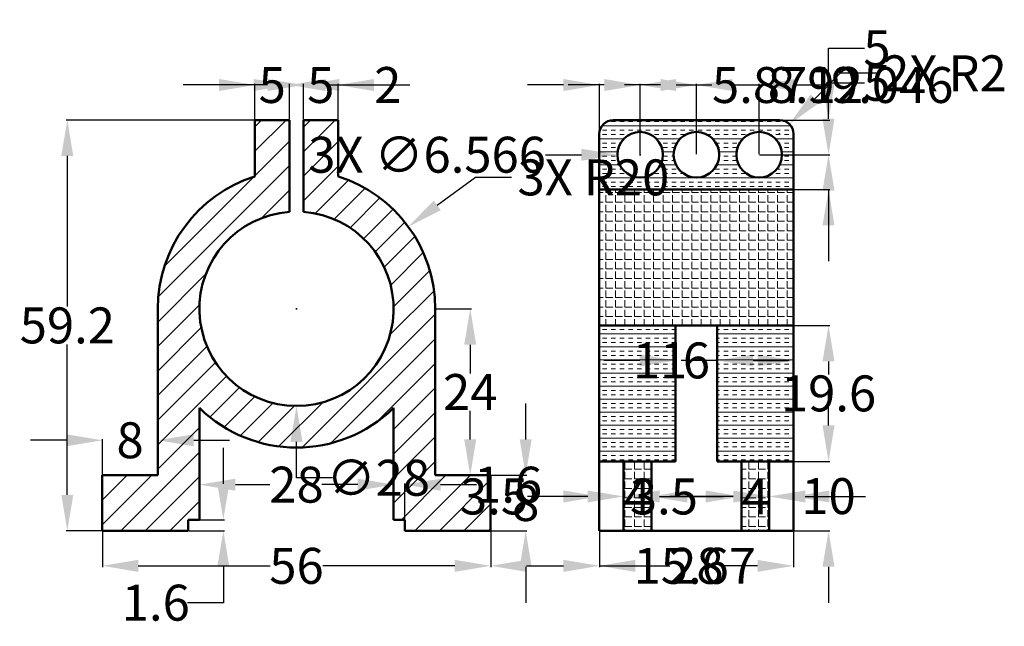
# Model space of a CAD drawing. Units: millimetres. Extents: x 58 to 200, y 31 to 118.
import ezdxf

# ---------------------------------------------------------------- set-up
doc = ezdxf.new("R2010")
doc.units = ezdxf.units.MM
doc.header["$MEASUREMENT"] = 0
for name, color, linetype, lineweight in [('M-DIMS', 2, 'Continuous', 18), ('M-HATC', 252, 'Continuous', 18), ('M-OUTL', 7, 'Continuous', 50)]:
    doc.layers.add(name, color=color, linetype=linetype, lineweight=lineweight)
doc.styles.get("Standard").update_dxf_attribs({"font": 'arial.ttf'})
doc.dimstyles.get("Standard").update_dxf_attribs({"dimtxt": 5.18, "dimasz": 5.18, "dimexe": 0.18, "dimexo": 0.0625, "dimgap": 0.09, "dimtad": 0, "dimtih": 1, "dimtoh": 1, "dimdec": 1, "dimzin": 0, "dimdsep": 46, "dimtxsty": 'Standard', "dimcen": 0.09, "dimadec": 0, "dimazin": 0, "dimtfac": 1, "dimtdec": 1, "dimtofl": 0, "dimtmove": 0, "dimatfit": 3, "dimfxl": 1, "dimtolj": 1, "dimtzin": 0, "dimarcsym": 0})

# ---------------------------------------------------------------- blocks, each defined once
blk = doc.blocks.new('*D1')
at = {"layer": 'Defpoints', "color": 0, "transparency": 16777216}
for p in [(70.39, 44.76), (126.39, 44.76), (126.39, 39.71)]:
    blk.add_point(p, dxfattribs=at)
at = {"layer": 'M-DIMS', "color": 0, "lineweight": -2, "transparency": 16777216}
for p, q in [((70.39, 44.69), (70.39, 39.53)), ((126.39, 44.69), (126.39, 39.53)), ((75.57, 39.71), (94.59, 39.71)), ((121.21, 39.71), (102.18, 39.71))]:
    blk.add_line(p, q, dxfattribs=at)
at = {"layer": 'M-DIMS', "color": 0, "transparency": 16777216}
for points in [[(75.57, 40.57), (75.57, 38.84), (70.39, 39.71)], [(121.21, 40.57), (121.21, 38.84), (126.39, 39.71)]]:
    blk.add_solid(points, dxfattribs=at)
at = {"layer": 'M-DIMS', "color": 0, "transparency": 16777216, "insert": (98.39, 39.71), "char_height": 5.18, "attachment_point": 5}
blk.add_mtext('\\A1;56', dxfattribs=at)
blk = doc.blocks.new('*D2')
at = {"layer": 'Defpoints', "color": 0, "transparency": 16777216}
for p in [(65.34, 103.96), (92.39, 103.96), (70.39, 44.76)]:
    blk.add_point(p, dxfattribs=at)
at = {"layer": 'M-DIMS', "color": 0, "lineweight": -2, "transparency": 16777216}
for p, q in [((92.32, 103.96), (65.16, 103.96)), ((65.34, 98.78), (65.34, 77.09)), ((65.34, 49.94), (65.34, 71.62)), ((70.32, 44.76), (65.16, 44.76))]:
    blk.add_line(p, q, dxfattribs=at)
at = {"layer": 'M-DIMS', "color": 0, "transparency": 16777216}
for points in [[(64.47, 98.78), (66.2, 98.78), (65.34, 103.96)], [(64.47, 49.94), (66.2, 49.94), (65.34, 44.76)]]:
    blk.add_solid(points, dxfattribs=at)
at = {"layer": 'M-DIMS', "color": 0, "transparency": 16777216, "insert": (65.34, 74.36), "char_height": 5.18, "attachment_point": 5}
blk.add_mtext('\\A1;59.2', dxfattribs=at)
blk = doc.blocks.new('*D3')
at = {"layer": 'Defpoints', "color": 0, "transparency": 16777216}
for p in [(118.39, 76.76), (118.39, 52.76), (123.44, 52.76)]:
    blk.add_point(p, dxfattribs=at)
at = {"layer": 'M-DIMS', "color": 0, "lineweight": -2, "transparency": 16777216}
for p, q in [((118.45, 76.76), (123.62, 76.76)), ((123.44, 71.58), (123.44, 67.45)), ((123.44, 57.94), (123.44, 62.07)), ((118.45, 52.76), (123.62, 52.76))]:
    blk.add_line(p, q, dxfattribs=at)
at = {"layer": 'M-DIMS', "color": 0, "transparency": 16777216}
for points in [[(122.57, 71.58), (124.3, 71.58), (123.44, 76.76)], [(122.57, 57.94), (124.3, 57.94), (123.44, 52.76)]]:
    blk.add_solid(points, dxfattribs=at)
at = {"layer": 'M-DIMS', "color": 0, "transparency": 16777216, "insert": (123.44, 64.76), "char_height": 5.18, "attachment_point": 5}
blk.add_mtext('\\A1;24', dxfattribs=at)
blk = doc.blocks.new('*D4')
at = {"layer": 'Defpoints', "color": 0, "transparency": 16777216}
for p in [(126.39, 52.76), (126.39, 44.76), (131.44, 44.76)]:
    blk.add_point(p, dxfattribs=at)
at = {"layer": 'M-DIMS', "color": 0, "lineweight": -2, "transparency": 16777216}
for p, q in [((131.44, 57.94), (131.44, 63.12)), ((126.45, 52.76), (131.62, 52.76)), ((126.45, 44.76), (131.62, 44.76)), ((131.44, 39.58), (131.44, 34.4))]:
    blk.add_line(p, q, dxfattribs=at)
at = {"layer": 'M-DIMS', "color": 0, "transparency": 16777216}
for points in [[(130.57, 57.94), (132.3, 57.94), (131.44, 52.76)], [(130.57, 39.58), (132.3, 39.58), (131.44, 44.76)]]:
    blk.add_solid(points, dxfattribs=at)
at = {"layer": 'M-DIMS', "color": 0, "transparency": 16777216, "insert": (131.44, 48.76), "char_height": 5.18, "attachment_point": 5}
blk.add_mtext('\\A1;8', dxfattribs=at)
blk = doc.blocks.new('*D5')
at = {"layer": 'Defpoints', "color": 0, "transparency": 16777216}
for p in [(82.79, 46.36), (82.79, 44.76), (87.84, 44.76)]:
    blk.add_point(p, dxfattribs=at)
at = {"layer": 'M-DIMS', "color": 0, "lineweight": -2, "transparency": 16777216}
for p, q in [((87.84, 51.54), (87.84, 56.72)), ((82.85, 46.36), (88.02, 46.36)), ((82.85, 44.76), (88.02, 44.76)), ((87.84, 39.58), (87.84, 34.4)), ((87.84, 34.4), (82.66, 34.4))]:
    blk.add_line(p, q, dxfattribs=at)
at = {"layer": 'M-DIMS', "color": 0, "transparency": 16777216}
for points in [[(86.97, 51.54), (88.7, 51.54), (87.84, 46.36)], [(86.97, 39.58), (88.7, 39.58), (87.84, 44.76)]]:
    blk.add_solid(points, dxfattribs=at)
at = {"layer": 'M-DIMS', "color": 0, "transparency": 16777216, "insert": (78.1, 34.4), "char_height": 5.18, "attachment_point": 5}
blk.add_mtext('\\A1;1.6', dxfattribs=at)
blk = doc.blocks.new('*D6')
at = {"layer": 'Defpoints', "color": 0, "transparency": 16777216}
for p in [(78.39, 57.81), (70.39, 52.76), (78.39, 52.76)]:
    blk.add_point(p, dxfattribs=at)
at = {"layer": 'M-DIMS', "color": 0, "lineweight": -2, "transparency": 16777216}
for p, q in [((65.21, 57.81), (60.03, 57.81)), ((70.39, 52.82), (70.39, 57.99)), ((78.39, 52.82), (78.39, 57.99)), ((83.57, 57.81), (88.75, 57.81))]:
    blk.add_line(p, q, dxfattribs=at)
at = {"layer": 'M-DIMS', "color": 0, "transparency": 16777216}
for points in [[(65.21, 58.67), (65.21, 56.94), (70.39, 57.81)], [(83.57, 58.67), (83.57, 56.94), (78.39, 57.81)]]:
    blk.add_solid(points, dxfattribs=at)
at = {"layer": 'M-DIMS', "color": 0, "transparency": 16777216, "insert": (74.39, 57.81), "char_height": 5.18, "attachment_point": 5}
blk.add_mtext('\\A1;8', dxfattribs=at)
blk = doc.blocks.new('*D7')
at = {"layer": 'Defpoints', "color": 0, "transparency": 16777216}
for p in [(112.39, 51.41), (84.39, 46.36), (112.39, 46.36)]:
    blk.add_point(p, dxfattribs=at)
at = {"layer": 'M-DIMS', "color": 0, "lineweight": -2, "transparency": 16777216}
for p, q in [((84.39, 46.42), (84.39, 51.59)), ((89.57, 51.41), (94.54, 51.41)), ((107.21, 51.41), (102.24, 51.41)), ((112.39, 46.42), (112.39, 51.59))]:
    blk.add_line(p, q, dxfattribs=at)
at = {"layer": 'M-DIMS', "color": 0, "transparency": 16777216}
for points in [[(89.57, 52.27), (89.57, 50.54), (84.39, 51.41)], [(107.21, 52.27), (107.21, 50.54), (112.39, 51.41)]]:
    blk.add_solid(points, dxfattribs=at)
at = {"layer": 'M-DIMS', "color": 0, "transparency": 16777216, "insert": (98.39, 51.41), "char_height": 5.18, "attachment_point": 5}
blk.add_mtext('\\A1;28', dxfattribs=at)
blk = doc.blocks.new('*D8')
at = {"layer": 'Defpoints', "color": 0, "transparency": 16777216}
for p in [(113.99, 51.41), (112.39, 46.36), (113.99, 46.36)]:
    blk.add_point(p, dxfattribs=at)
at = {"layer": 'M-DIMS', "color": 0, "lineweight": -2, "transparency": 16777216}
for p, q in [((107.21, 51.41), (102.03, 51.41)), ((112.39, 46.42), (112.39, 51.59)), ((113.99, 46.42), (113.99, 51.59)), ((119.17, 51.41), (124.35, 51.41))]:
    blk.add_line(p, q, dxfattribs=at)
at = {"layer": 'M-DIMS', "color": 0, "transparency": 16777216}
for points in [[(107.21, 52.27), (107.21, 50.54), (112.39, 51.41)], [(119.17, 52.27), (119.17, 50.54), (113.99, 51.41)]]:
    blk.add_solid(points, dxfattribs=at)
at = {"layer": 'M-DIMS', "color": 0, "transparency": 16777216, "insert": (128.91, 51.41), "char_height": 5.18, "attachment_point": 5}
blk.add_mtext('\\A1;1.6', dxfattribs=at)
blk = doc.blocks.new('*D9')
at = {"layer": 'Defpoints', "color": 0, "transparency": 16777216}
for p in [(97.39, 109.01), (92.39, 103.96), (97.39, 103.96)]:
    blk.add_point(p, dxfattribs=at)
at = {"layer": 'M-DIMS', "color": 0, "lineweight": -2, "transparency": 16777216}
for p, q in [((87.21, 109.01), (82.03, 109.01)), ((92.39, 104.02), (92.39, 109.19)), ((97.39, 104.02), (97.39, 109.19)), ((102.57, 109.01), (107.75, 109.01))]:
    blk.add_line(p, q, dxfattribs=at)
at = {"layer": 'M-DIMS', "color": 0, "transparency": 16777216}
for points in [[(87.21, 109.87), (87.21, 108.14), (92.39, 109.01)], [(102.57, 109.87), (102.57, 108.14), (97.39, 109.01)]]:
    blk.add_solid(points, dxfattribs=at)
at = {"layer": 'M-DIMS', "color": 0, "transparency": 16777216, "insert": (94.89, 109.01), "char_height": 5.18, "attachment_point": 5}
blk.add_mtext('\\A1;5', dxfattribs=at)
blk = doc.blocks.new('*D10')
at = {"layer": 'Defpoints', "color": 0, "transparency": 16777216}
for p in [(99.39, 109.01), (97.39, 103.96), (99.39, 103.96)]:
    blk.add_point(p, dxfattribs=at)
at = {"layer": 'M-DIMS', "color": 0, "lineweight": -2, "transparency": 16777216}
for p, q in [((92.21, 109.01), (87.03, 109.01)), ((97.39, 104.02), (97.39, 109.19)), ((99.39, 104.02), (99.39, 109.19)), ((104.57, 109.01), (109.75, 109.01))]:
    blk.add_line(p, q, dxfattribs=at)
at = {"layer": 'M-DIMS', "color": 0, "transparency": 16777216}
for points in [[(92.21, 109.87), (92.21, 108.14), (97.39, 109.01)], [(104.57, 109.87), (104.57, 108.14), (99.39, 109.01)]]:
    blk.add_solid(points, dxfattribs=at)
at = {"layer": 'M-DIMS', "color": 0, "transparency": 16777216, "insert": (111.55, 109.01), "char_height": 5.18, "attachment_point": 5}
blk.add_mtext('\\A1;2', dxfattribs=at)
blk = doc.blocks.new('*D11')
at = {"layer": 'Defpoints', "color": 0, "transparency": 16777216}
for p in [(104.39, 109.01), (99.39, 103.96), (104.39, 103.96)]:
    blk.add_point(p, dxfattribs=at)
at = {"layer": 'M-DIMS', "color": 0, "lineweight": -2, "transparency": 16777216}
for p, q in [((94.21, 109.01), (89.03, 109.01)), ((99.39, 104.02), (99.39, 109.19)), ((104.39, 104.02), (104.39, 109.19)), ((109.57, 109.01), (114.75, 109.01))]:
    blk.add_line(p, q, dxfattribs=at)
at = {"layer": 'M-DIMS', "color": 0, "transparency": 16777216}
for points in [[(94.21, 109.87), (94.21, 108.14), (99.39, 109.01)], [(109.57, 109.87), (109.57, 108.14), (104.39, 109.01)]]:
    blk.add_solid(points, dxfattribs=at)
at = {"layer": 'M-DIMS', "color": 0, "transparency": 16777216, "insert": (101.89, 109.01), "char_height": 5.18, "attachment_point": 5}
blk.add_mtext('\\A1;5', dxfattribs=at)
blk = doc.blocks.new('*D12')
at = {"layer": 'Defpoints', "color": 0, "transparency": 16777216}
for p in [(142.06, 44.76), (170.06, 44.76), (170.06, 39.71)]:
    blk.add_point(p, dxfattribs=at)
at = {"layer": 'M-DIMS', "color": 0, "lineweight": -2, "transparency": 16777216}
for p, q in [((142.06, 44.69), (142.06, 39.53)), ((170.06, 44.69), (170.06, 39.53)), ((147.24, 39.71), (152.21, 39.71)), ((164.88, 39.71), (159.91, 39.71))]:
    blk.add_line(p, q, dxfattribs=at)
at = {"layer": 'M-DIMS', "color": 0, "transparency": 16777216}
for points in [[(147.24, 40.57), (147.24, 38.84), (142.06, 39.71)], [(164.88, 40.57), (164.88, 38.84), (170.06, 39.71)]]:
    blk.add_solid(points, dxfattribs=at)
at = {"layer": 'M-DIMS', "color": 0, "transparency": 16777216, "insert": (156.06, 39.71), "char_height": 5.18, "attachment_point": 5}
blk.add_mtext('\\A1;28', dxfattribs=at)
blk = doc.blocks.new('*D13')
at = {"layer": 'Defpoints', "color": 0, "transparency": 16777216}
for p in [(153.06, 74.36), (159.06, 74.36), (153.06, 69.31)]:
    blk.add_point(p, dxfattribs=at)
at = {"layer": 'M-DIMS', "color": 0, "lineweight": -2, "transparency": 16777216}
for p, q in [((153.06, 74.29), (153.06, 69.13)), ((159.06, 74.29), (159.06, 69.13)), ((147.88, 69.31), (142.7, 69.31)), ((164.24, 69.31), (169.42, 69.31))]:
    blk.add_line(p, q, dxfattribs=at)
at = {"layer": 'M-DIMS', "color": 0, "transparency": 16777216}
for points in [[(147.88, 70.17), (147.88, 68.44), (153.06, 69.31)], [(164.24, 70.17), (164.24, 68.44), (159.06, 69.31)]]:
    blk.add_solid(points, dxfattribs=at)
at = {"layer": 'M-DIMS', "color": 0, "transparency": 16777216, "insert": (156.06, 69.31), "char_height": 5.18, "attachment_point": 5}
blk.add_mtext('\\A1;6', dxfattribs=at)
blk = doc.blocks.new('*D14')
at = {"layer": 'Defpoints', "color": 0, "transparency": 16777216}
for p in [(159.06, 74.36), (170.06, 74.36), (159.06, 69.31)]:
    blk.add_point(p, dxfattribs=at)
at = {"layer": 'M-DIMS', "color": 0, "lineweight": -2, "transparency": 16777216}
for p, q in [((159.06, 74.29), (159.06, 69.13)), ((170.06, 74.29), (170.06, 69.13)), ((159.06, 69.31), (153.88, 69.31)), ((164.88, 69.31), (164.24, 69.31))]:
    blk.add_line(p, q, dxfattribs=at)
at = {"layer": 'M-DIMS', "color": 0, "transparency": 16777216}
for points in [[(164.24, 70.17), (164.24, 68.44), (159.06, 69.31)], [(164.88, 70.17), (164.88, 68.44), (170.06, 69.31)]]:
    blk.add_solid(points, dxfattribs=at)
at = {"layer": 'M-DIMS', "color": 0, "transparency": 16777216, "insert": (150.82, 69.31), "char_height": 5.18, "attachment_point": 5}
blk.add_mtext('\\A1;11', dxfattribs=at)
blk = doc.blocks.new('*D15')
at = {"layer": 'Defpoints', "color": 0, "transparency": 16777216}
for p in [(142.06, 54.76), (145.56, 54.76), (142.06, 49.71)]:
    blk.add_point(p, dxfattribs=at)
at = {"layer": 'M-DIMS', "color": 0, "lineweight": -2, "transparency": 16777216}
for p, q in [((142.06, 54.69), (142.06, 49.53)), ((145.56, 54.69), (145.56, 49.53)), ((136.88, 49.71), (131.7, 49.71)), ((150.74, 49.71), (155.92, 49.71))]:
    blk.add_line(p, q, dxfattribs=at)
at = {"layer": 'M-DIMS', "color": 0, "transparency": 16777216}
for points in [[(136.88, 50.57), (136.88, 48.84), (142.06, 49.71)], [(150.74, 50.57), (150.74, 48.84), (145.56, 49.71)]]:
    blk.add_solid(points, dxfattribs=at)
at = {"layer": 'M-DIMS', "color": 0, "transparency": 16777216, "insert": (126.87, 49.71), "char_height": 5.18, "attachment_point": 5}
blk.add_mtext('\\A1;3.5', dxfattribs=at)
blk = doc.blocks.new('*D16')
at = {"layer": 'Defpoints', "color": 0, "transparency": 16777216}
for p in [(145.56, 54.76), (149.56, 54.76), (145.56, 49.71)]:
    blk.add_point(p, dxfattribs=at)
at = {"layer": 'M-DIMS', "color": 0, "lineweight": -2, "transparency": 16777216}
for p, q in [((145.56, 54.69), (145.56, 49.53)), ((149.56, 54.69), (149.56, 49.53)), ((140.38, 49.71), (135.2, 49.71)), ((154.74, 49.71), (159.92, 49.71))]:
    blk.add_line(p, q, dxfattribs=at)
at = {"layer": 'M-DIMS', "color": 0, "transparency": 16777216}
for points in [[(140.38, 50.57), (140.38, 48.84), (145.56, 49.71)], [(154.74, 50.57), (154.74, 48.84), (149.56, 49.71)]]:
    blk.add_solid(points, dxfattribs=at)
at = {"layer": 'M-DIMS', "color": 0, "transparency": 16777216, "insert": (147.56, 49.71), "char_height": 5.18, "attachment_point": 5}
blk.add_mtext('\\A1;4', dxfattribs=at)
blk = doc.blocks.new('*D17')
at = {"layer": 'Defpoints', "color": 0, "transparency": 16777216}
for p in [(170.06, 54.76), (175.11, 54.76), (170.06, 44.76)]:
    blk.add_point(p, dxfattribs=at)
at = {"layer": 'M-DIMS', "color": 0, "lineweight": -2, "transparency": 16777216}
for p, q in [((175.11, 59.94), (175.11, 65.12)), ((170.12, 54.76), (175.29, 54.76)), ((170.12, 44.76), (175.29, 44.76)), ((175.11, 39.58), (175.11, 34.4))]:
    blk.add_line(p, q, dxfattribs=at)
at = {"layer": 'M-DIMS', "color": 0, "transparency": 16777216}
for points in [[(174.24, 59.94), (175.97, 59.94), (175.11, 54.76)], [(174.24, 39.58), (175.97, 39.58), (175.11, 44.76)]]:
    blk.add_solid(points, dxfattribs=at)
at = {"layer": 'M-DIMS', "color": 0, "transparency": 16777216, "insert": (175.11, 49.76), "char_height": 5.18, "attachment_point": 5}
blk.add_mtext('\\A1;10', dxfattribs=at)
blk = doc.blocks.new('*D18')
at = {"layer": 'Defpoints', "color": 0, "transparency": 16777216}
for p in [(170.06, 74.36), (175.11, 74.36), (170.06, 54.76)]:
    blk.add_point(p, dxfattribs=at)
at = {"layer": 'M-DIMS', "color": 0, "lineweight": -2, "transparency": 16777216}
for p, q in [((170.12, 74.36), (175.29, 74.36)), ((175.11, 69.18), (175.11, 67.29)), ((175.11, 59.94), (175.11, 61.82)), ((170.12, 54.76), (175.29, 54.76))]:
    blk.add_line(p, q, dxfattribs=at)
at = {"layer": 'M-DIMS', "color": 0, "transparency": 16777216}
for points in [[(174.24, 69.18), (175.97, 69.18), (175.11, 74.36)], [(174.24, 59.94), (175.97, 59.94), (175.11, 54.76)]]:
    blk.add_solid(points, dxfattribs=at)
at = {"layer": 'M-DIMS', "color": 0, "transparency": 16777216, "insert": (175.11, 64.56), "char_height": 5.18, "attachment_point": 5}
blk.add_mtext('\\A1;19.6', dxfattribs=at)
blk = doc.blocks.new('*D19')
at = {"layer": 'Defpoints', "color": 0, "transparency": 16777216}
for p in [(165.1, 98.96), (175.11, 98.96), (170.06, 93.96)]:
    blk.add_point(p, dxfattribs=at)
at = {"layer": 'M-DIMS', "color": 0, "lineweight": -2, "transparency": 16777216}
for p, q in [((175.11, 104.14), (175.11, 109.32)), ((175.11, 109.32), (180.29, 109.32)), ((165.16, 98.96), (175.29, 98.96)), ((170.12, 93.96), (175.29, 93.96)), ((175.11, 88.78), (175.11, 83.6))]:
    blk.add_line(p, q, dxfattribs=at)
at = {"layer": 'M-DIMS', "color": 0, "transparency": 16777216}
for points in [[(174.24, 104.14), (175.97, 104.14), (175.11, 98.96)], [(174.24, 88.78), (175.97, 88.78), (175.11, 93.96)]]:
    blk.add_solid(points, dxfattribs=at)
at = {"layer": 'M-DIMS', "color": 0, "transparency": 16777216, "insert": (182.09, 109.32), "char_height": 5.18, "attachment_point": 5}
blk.add_mtext('\\A1;5', dxfattribs=at)
blk = doc.blocks.new('*D20')
at = {"layer": 'Defpoints', "color": 0, "transparency": 16777216}
for p in [(168.06, 103.96), (175.11, 103.96), (165.1, 98.96)]:
    blk.add_point(p, dxfattribs=at)
at = {"layer": 'M-DIMS', "color": 0, "lineweight": -2, "transparency": 16777216}
for p, q in [((175.11, 109.14), (175.11, 114.32)), ((175.11, 114.32), (180.29, 114.32)), ((168.12, 103.96), (175.29, 103.96)), ((165.16, 98.96), (175.29, 98.96)), ((175.11, 93.78), (175.11, 88.6))]:
    blk.add_line(p, q, dxfattribs=at)
at = {"layer": 'M-DIMS', "color": 0, "transparency": 16777216}
for points in [[(174.24, 109.14), (175.97, 109.14), (175.11, 103.96)], [(174.24, 93.78), (175.97, 93.78), (175.11, 98.96)]]:
    blk.add_solid(points, dxfattribs=at)
at = {"layer": 'M-DIMS', "color": 0, "transparency": 16777216, "insert": (182.09, 114.32), "char_height": 5.18, "attachment_point": 5}
blk.add_mtext('\\A1;5', dxfattribs=at)
blk = doc.blocks.new('*D21')
at = {"layer": 'Defpoints', "color": 0, "transparency": 16777216}
for p in [(147.94, 109.01), (142.06, 101.96), (147.94, 98.96)]:
    blk.add_point(p, dxfattribs=at)
at = {"layer": 'M-DIMS', "color": 0, "lineweight": -2, "transparency": 16777216}
for p, q in [((136.88, 109.01), (131.7, 109.01)), ((142.06, 102.02), (142.06, 109.19)), ((147.94, 99.02), (147.94, 109.19)), ((153.12, 109.01), (158.3, 109.01))]:
    blk.add_line(p, q, dxfattribs=at)
at = {"layer": 'M-DIMS', "color": 0, "transparency": 16777216}
for points in [[(136.88, 109.87), (136.88, 108.14), (142.06, 109.01)], [(153.12, 109.87), (153.12, 108.14), (147.94, 109.01)]]:
    blk.add_solid(points, dxfattribs=at)
at = {"layer": 'M-DIMS', "color": 0, "transparency": 16777216, "insert": (167.13, 109.01), "char_height": 5.18, "attachment_point": 5}
blk.add_mtext('\\A1;5.879', dxfattribs=at)
blk = doc.blocks.new('*D22')
at = {"layer": 'Defpoints', "color": 0, "transparency": 16777216}
for p in [(156.06, 109.01), (147.94, 98.96), (156.06, 98.96)]:
    blk.add_point(p, dxfattribs=at)
at = {"layer": 'M-DIMS', "color": 0, "lineweight": -2, "transparency": 16777216}
for p, q in [((142.76, 109.01), (137.58, 109.01)), ((147.94, 99.02), (147.94, 109.19)), ((156.06, 99.02), (156.06, 109.19)), ((161.24, 109.01), (166.42, 109.01))]:
    blk.add_line(p, q, dxfattribs=at)
at = {"layer": 'M-DIMS', "color": 0, "transparency": 16777216}
for points in [[(142.76, 109.87), (142.76, 108.14), (147.94, 109.01)], [(161.24, 109.87), (161.24, 108.14), (156.06, 109.01)]]:
    blk.add_solid(points, dxfattribs=at)
at = {"layer": 'M-DIMS', "color": 0, "transparency": 16777216, "insert": (173.21, 109.01), "char_height": 5.18, "attachment_point": 5}
blk.add_mtext('\\A1;8.12', dxfattribs=at)
blk = doc.blocks.new('*D23')
at = {"layer": 'Defpoints', "color": 0, "transparency": 16777216}
for p in [(165.1, 109.01), (156.06, 98.96), (165.1, 98.96)]:
    blk.add_point(p, dxfattribs=at)
at = {"layer": 'M-DIMS', "color": 0, "lineweight": -2, "transparency": 16777216}
for p, q in [((150.88, 109.01), (145.7, 109.01)), ((156.06, 99.02), (156.06, 109.19)), ((165.1, 99.02), (165.1, 109.19)), ((170.28, 109.01), (175.46, 109.01))]:
    blk.add_line(p, q, dxfattribs=at)
at = {"layer": 'M-DIMS', "color": 0, "transparency": 16777216}
for points in [[(150.88, 109.87), (150.88, 108.14), (156.06, 109.01)], [(170.28, 109.87), (170.28, 108.14), (165.1, 109.01)]]:
    blk.add_solid(points, dxfattribs=at)
at = {"layer": 'M-DIMS', "color": 0, "transparency": 16777216, "insert": (184.29, 109.01), "char_height": 5.18, "attachment_point": 5}
blk.add_mtext('\\A1;9.046', dxfattribs=at)
blk = doc.blocks.new('*D24')
at = {"layer": 'Defpoints', "color": 0, "transparency": 16777216}
for p in [(126.39, 44.76), (142.06, 44.76), (142.06, 39.71)]:
    blk.add_point(p, dxfattribs=at)
at = {"layer": 'M-DIMS', "color": 0, "lineweight": -2, "transparency": 16777216}
for p, q in [((126.39, 44.69), (126.39, 39.53)), ((142.06, 44.69), (142.06, 39.53)), ((131.57, 39.71), (136.88, 39.71)), ((142.06, 39.71), (147.24, 39.71))]:
    blk.add_line(p, q, dxfattribs=at)
at = {"layer": 'M-DIMS', "color": 0, "transparency": 16777216}
for points in [[(131.57, 40.57), (131.57, 38.84), (126.39, 39.71)], [(136.88, 40.57), (136.88, 38.84), (142.06, 39.71)]]:
    blk.add_solid(points, dxfattribs=at)
at = {"layer": 'M-DIMS', "color": 0, "transparency": 16777216, "insert": (155.82, 39.71), "char_height": 5.18, "attachment_point": 5}
blk.add_mtext('\\A1;15.67', dxfattribs=at)
blk = doc.blocks.new('*D25')
at = {"layer": 'Defpoints', "color": 0, "transparency": 16777216}
for p in [(162.56, 54.76), (166.56, 54.76), (162.56, 49.71)]:
    blk.add_point(p, dxfattribs=at)
at = {"layer": 'M-DIMS', "color": 0, "lineweight": -2, "transparency": 16777216}
for p, q in [((162.56, 54.69), (162.56, 49.53)), ((166.56, 54.69), (166.56, 49.53)), ((157.38, 49.71), (152.2, 49.71)), ((171.74, 49.71), (176.92, 49.71))]:
    blk.add_line(p, q, dxfattribs=at)
at = {"layer": 'M-DIMS', "color": 0, "transparency": 16777216}
for points in [[(157.38, 50.57), (157.38, 48.84), (162.56, 49.71)], [(171.74, 50.57), (171.74, 48.84), (166.56, 49.71)]]:
    blk.add_solid(points, dxfattribs=at)
at = {"layer": 'M-DIMS', "color": 0, "transparency": 16777216, "insert": (164.56, 49.71), "char_height": 5.18, "attachment_point": 5}
blk.add_mtext('\\A1;4', dxfattribs=at)
blk = doc.blocks.new('*D26')
at = {"layer": 'Defpoints', "color": 0, "transparency": 16777216}
for p in [(166.56, 54.76), (170.06, 54.76), (166.56, 49.71)]:
    blk.add_point(p, dxfattribs=at)
at = {"layer": 'M-DIMS', "color": 0, "lineweight": -2, "transparency": 16777216}
for p, q in [((166.56, 54.69), (166.56, 49.53)), ((170.06, 54.69), (170.06, 49.53)), ((161.38, 49.71), (156.2, 49.71)), ((175.24, 49.71), (180.42, 49.71))]:
    blk.add_line(p, q, dxfattribs=at)
at = {"layer": 'M-DIMS', "color": 0, "transparency": 16777216}
for points in [[(161.38, 50.57), (161.38, 48.84), (166.56, 49.71)], [(175.24, 50.57), (175.24, 48.84), (170.06, 49.71)]]:
    blk.add_solid(points, dxfattribs=at)
at = {"layer": 'M-DIMS', "color": 0, "transparency": 16777216, "insert": (151.37, 49.71), "char_height": 5.18, "attachment_point": 5}
blk.add_mtext('\\A1;3.5', dxfattribs=at)
blk = doc.blocks.new('*D27')
at = {"layer": 'Defpoints', "color": 0, "transparency": 16777216}
for p in [(98.39, 90.76), (98.39, 62.76)]:
    blk.add_point(p, dxfattribs=at)
at = {"layer": 'M-DIMS', "color": 0, "lineweight": -2, "transparency": 16777216}
for p, q in [((98.3, 76.76), (98.48, 76.76)), ((98.39, 76.67), (98.39, 76.85)), ((98.39, 52.4), (98.39, 57.58)), ((103.57, 52.4), (98.39, 52.4))]:
    blk.add_line(p, q, dxfattribs=at)
at = {"layer": 'M-DIMS', "color": 0, "transparency": 16777216}
blk.add_solid([(99.25, 57.58), (97.52, 57.58), (98.39, 62.76)], dxfattribs=at)
at = {"layer": 'M-DIMS', "color": 0, "transparency": 16777216, "insert": (110.19, 52.4), "char_height": 5.18, "attachment_point": 5}
blk.add_mtext('\\A1;∅28', dxfattribs=at)
blk = doc.blocks.new('*D28')
at = {"layer": 'Defpoints', "color": 0, "transparency": 16777216}
for p in [(114.51, 88.59), (98.39, 76.76)]:
    blk.add_point(p, dxfattribs=at)
at = {"layer": 'M-DIMS', "color": 0, "lineweight": -2, "transparency": 16777216}
for p, q in [((124.19, 95.69), (118.69, 91.65)), ((129.37, 95.69), (124.19, 95.69)), ((98.3, 76.76), (98.48, 76.76)), ((98.39, 76.67), (98.39, 76.85))]:
    blk.add_line(p, q, dxfattribs=at)
at = {"layer": 'M-DIMS', "color": 0, "transparency": 16777216}
blk.add_solid([(118.18, 92.35), (119.2, 90.96), (114.51, 88.59)], dxfattribs=at)
at = {"layer": 'M-DIMS', "color": 0, "transparency": 16777216, "insert": (141.2, 95.69), "char_height": 5.18, "attachment_point": 5}
blk.add_mtext('\\A1;3X R20', dxfattribs=at)
blk = doc.blocks.new('*D29')
at = {"layer": 'Defpoints', "color": 0, "transparency": 16777216}
for p in [(144.65, 98.96), (151.22, 98.96)]:
    blk.add_point(p, dxfattribs=at)
at = {"layer": 'M-DIMS', "color": 0, "lineweight": -2, "transparency": 16777216}
for p, q in [((134.29, 98.96), (139.47, 98.96)), ((147.85, 98.96), (148.03, 98.96)), ((147.94, 98.87), (147.94, 99.05))]:
    blk.add_line(p, q, dxfattribs=at)
at = {"layer": 'M-DIMS', "color": 0, "transparency": 16777216}
blk.add_solid([(139.47, 99.82), (139.47, 98.09), (144.65, 98.96)], dxfattribs=at)
at = {"layer": 'M-DIMS', "color": 0, "transparency": 16777216, "insert": (117.22, 98.96), "char_height": 5.18, "attachment_point": 5}
blk.add_mtext('\\A1;3X ∅6.566', dxfattribs=at)
blk = doc.blocks.new('*D30')
at = {"layer": 'Defpoints', "color": 0, "transparency": 16777216}
for p in [(169.47, 103.37), (168.06, 101.96)]:
    blk.add_point(p, dxfattribs=at)
at = {"layer": 'M-DIMS', "color": 0, "lineweight": -2, "transparency": 16777216}
for p, q in [((176.8, 110.69), (173.13, 107.03)), ((181.98, 110.69), (176.8, 110.69)), ((167.97, 101.96), (168.15, 101.96)), ((168.06, 101.87), (168.06, 102.05))]:
    blk.add_line(p, q, dxfattribs=at)
at = {"layer": 'M-DIMS', "color": 0, "transparency": 16777216}
blk.add_solid([(172.52, 107.64), (173.75, 106.42), (169.47, 103.37)], dxfattribs=at)
at = {"layer": 'M-DIMS', "color": 0, "transparency": 16777216, "insert": (191.83, 110.69), "char_height": 5.18, "attachment_point": 5}
blk.add_mtext('\\A1;2X R2', dxfattribs=at)

msp = doc.modelspace()

# ---------------------------------------------------------------- hatches: boundary and pattern name
at = {"layer": 'M-HATC'}
h = msp.add_hatch(dxfattribs=at)
h.set_pattern_fill('ANSI31', color=256, scale=20)
h.paths.add_polyline_path([(118.3866, 76.7562, 0.32753822), (104.3866, 95.835), (104.3866, 96.7562), (104.3866, 103.9562), (99.3866, 103.9562), (99.3866, 96.7562), (99.3866, 90.7204, -27.96424004), (97.3866, 90.7204), (97.3866, 90.7562), (97.3866, 96.7562), (97.3866, 103.9562), (92.3866, 103.9562), (92.3866, 96.7562), (92.3866, 95.835, 0.32753822), (78.3866, 76.7562), (78.3866, 52.7562), (74.3866, 52.7562), (70.3866, 52.7562), (70.3866, 48.7562), (70.3866, 44.7562), (82.7866, 44.7562), (82.7866, 46.3562), (84.3866, 46.3562), (84.3866, 52.7562), (84.3866, 62.4733, 0.40836737), (112.3866, 62.4733), (112.3866, 52.7562), (112.3866, 46.3562), (113.9866, 46.3562), (113.9866, 44.7562), (118.3866, 44.7562), (126.3866, 44.7562), (126.3866, 52.7562), (118.3866, 52.7562)])
h = msp.add_hatch(dxfattribs=at)
h.set_pattern_fill('INSUL', color=256, scale=5)
h.paths.add_polyline_path([(153.0567, 74.3562), (142.0567, 74.3562), (142.0567, 54.7562), (153.0567, 54.7562)])
h.paths.add_polyline_path([(170.0567, 74.3562), (159.0567, 74.3562), (159.0567, 54.7562), (170.0567, 54.7562)])
h.paths.add_polyline_path([(170.0567, 101.9562, 0.41421356), (168.0567, 103.9562), (144.0567, 103.9562, 0.41421356), (142.0567, 101.9562), (142.0567, 93.9562), (170.0567, 93.9562)])
h.paths.add_polyline_path([(152.7738, 98.9562, -1), (159.3395, 98.9562, -1)], flags=16)
h.paths.add_polyline_path([(144.6532, 98.9562, -1), (151.2189, 98.9562, -1)], flags=16)
h.paths.add_polyline_path([(161.8196, 98.9562, -1), (168.3853, 98.9562, -1)], flags=16)
h = msp.add_hatch(dxfattribs=at)
h.set_pattern_fill('ANGLE', color=256, scale=5)
h.set_pattern_definition([(0, (0, 0), (0, 1.375), [1, -0.375]), (90, (0, 0), (-1.375, 1e-16), [1, -0.375])])
h.paths.add_polyline_path([(170.0567, 93.9562), (142.0567, 93.9562), (142.0567, 74.3562), (170.0567, 74.3562)])
h.paths.add_polyline_path([(149.5567, 54.7562), (145.5567, 54.7562), (145.5567, 44.7562), (149.5567, 44.7562)])
h.paths.add_polyline_path([(166.5567, 54.7562), (162.5567, 54.7562), (162.5567, 44.7562), (166.5567, 44.7562)])

# ---------------------------------------------------------------- linework, layer by layer
at = {"layer": 'M-OUTL'}
for p, q in [((92.3866, 96.7562), (92.3866, 103.9562)), ((92.3866, 103.9562), (97.3866, 103.9562)), ((97.3866, 96.7562), (97.3866, 103.9562)), ((99.3866, 96.7562), (99.3866, 103.9562)), ((99.3866, 103.9562), (104.3866, 103.9562)), ((104.3866, 96.7562), (104.3866, 103.9562)), ((144.0567, 103.9562), (168.0567, 103.9562)), ((142.0567, 101.9562), (142.0567, 44.7562)), ((170.0567, 101.9562), (170.0567, 44.7562)), ((92.3866, 96.7562), (92.3866, 95.835)), ((97.3866, 96.7562), (97.3866, 90.7562)), ((99.3866, 96.7562), (99.3866, 90.7562)), ((104.3866, 96.7562), (104.3866, 95.835)), ((142.0567, 93.9562), (170.0567, 93.9562)), ((97.3866, 90.7562), (97.3866, 90.7204)), ((99.3866, 90.7562), (99.3866, 90.7204)), ((78.3866, 76.7562), (78.3866, 52.7562)), ((118.3866, 76.7562), (118.3866, 52.7562)), ((142.0567, 74.3562), (170.0567, 74.3562)), ((153.0567, 74.3562), (153.0567, 54.7562)), ((159.0567, 74.3562), (159.0567, 54.7562)), ((84.3866, 62.4733), (84.3866, 52.7562)), ((112.3866, 62.4733), (112.3866, 52.7562)), ((142.0567, 54.7562), (153.0567, 54.7562)), ((142.0567, 54.7562), (153.0567, 54.7562)), ((145.5567, 54.7562), (145.5567, 44.7562)), ((149.5567, 54.7562), (149.5567, 44.7562)), ((159.0567, 54.7562), (170.0567, 54.7562)), ((162.5567, 54.7562), (162.5567, 44.7562)), ((166.5567, 54.7562), (166.5567, 44.7562)), ((74.3866, 52.7562), (70.3866, 52.7562)), ((70.3866, 52.7562), (70.3866, 48.7562)), ((78.3866, 52.7562), (74.3866, 52.7562)), ((84.3866, 52.7562), (84.3866, 46.3562)), ((112.3866, 52.7562), (112.3866, 46.3562)), ((126.3866, 52.7562), (118.3866, 52.7562)), ((126.3866, 44.7562), (126.3866, 52.7562)), ((70.3866, 48.7562), (70.3866, 44.7562)), ((84.3866, 46.3562), (82.7866, 46.3562)), ((82.7866, 46.3562), (82.7866, 44.7562)), ((113.9866, 46.3562), (112.3866, 46.3562)), ((113.9866, 46.3562), (113.9866, 44.7562)), ((70.3866, 44.7562), (82.7866, 44.7562)), ((113.9866, 44.7562), (118.3866, 44.7562)), ((118.3866, 44.7562), (126.3866, 44.7562)), ((142.0567, 44.7562), (170.0567, 44.7562))]:
    msp.add_line(p, q, dxfattribs=at)
for centre in [(147.936, 98.9562), (156.0567, 98.9562), (165.1025, 98.9562)]:
    msp.add_circle(centre, 3.2828, dxfattribs=at)
for centre, radius, start, end in [((144.0567, 101.9562), 2, 90, 180), ((168.0567, 101.9562), 2, 0, 90), ((98.3866, 76.7562), 20, 107.457603, 180), ((98.3866, 76.7562), 20, 0, 72.542397), ((98.3866, 76.7562), 14, 94.096044, 85.903956), ((98.3866, 76.7562), 20, 225.572996, 314.427004)]:
    msp.add_arc(centre, radius, start, end, dxfattribs=at)

# ---------------------------------------------------------------- dimensions: what is measured, and where the dimension line sits
at = {"layer": 'M-DIMS'}
dim = msp.add_radius_dim(center=(168.0567, 101.9562), mpoint=(169.4712, 103.3702), text='2X <>', dimstyle='Standard', override={"dimdec": 0, "dimlfac": 1, "dimrnd": 0, "dimzin": 0, "dimdsep": 46, "dimlunit": 2}, dxfattribs=at)
dim.commit()
dim.dimension.update_dxf_attribs({"geometry": '*D30', "text_midpoint": (191.8275, 110.6944)})
for base, p1, p2, angle, override, picture, middle in [((175.1067, 103.9562), (165.1025, 98.9562), (168.0567, 103.9562), 90, {"dimdec": 0, "dimlfac": 1, "dimrnd": 0, "dimzin": 0, "dimdsep": 46, "dimlunit": 2}, '*D20', (182.0939, 114.3162)), ((175.1067, 98.9562), (170.0567, 93.9562), (165.1025, 98.9562), 90, {"dimdec": 0, "dimlfac": 1, "dimrnd": 0, "dimzin": 0, "dimdsep": 46, "dimlunit": 2}, '*D19', (182.0939, 109.3162)), ((65.3366, 103.9562), (70.3866, 44.7562), (92.3866, 103.9562), 90, {"dimdec": 1, "dimlfac": 1, "dimrnd": 0, "dimzin": 0, "dimdsep": 46, "dimlunit": 2}, '*D2', (65.3366, 74.3562)), ((123.4366, 52.7562), (118.3866, 76.7562), (118.3866, 52.7562), 270, {"dimdec": 0, "dimlfac": 1, "dimrnd": 0, "dimzin": 0, "dimdsep": 46, "dimlunit": 2}, '*D3', (123.4366, 64.7562)), ((153.0567, 69.3062), (159.0567, 74.3562), (153.0567, 74.3562), 180, {"dimdec": 0, "dimlfac": 1, "dimrnd": 0, "dimzin": 0, "dimdsep": 46, "dimlunit": 2}, '*D13', (156.0567, 69.3062)), ((159.0567, 69.3062), (170.0567, 74.3562), (159.0567, 74.3562), 180, {"dimdec": 0, "dimlfac": 1, "dimrnd": 0, "dimzin": 0, "dimdsep": 46, "dimlunit": 2}, '*D14', (150.8204, 69.3062)), ((175.1067, 74.3562), (170.0567, 54.7562), (170.0567, 74.3562), 90, {"dimdec": 1, "dimlfac": 1, "dimrnd": 0, "dimzin": 0, "dimdsep": 46, "dimlunit": 2}, '*D18', (175.1067, 64.5562)), ((175.1067, 54.7562), (170.0567, 44.7562), (170.0567, 54.7562), 90, {"dimdec": 0, "dimlfac": 1, "dimrnd": 0, "dimzin": 0, "dimdsep": 46, "dimlunit": 2}, '*D17', (175.1067, 49.7562)), ((131.4366, 44.7562), (126.3866, 52.7562), (126.3866, 44.7562), 270, {"dimdec": 0, "dimlfac": 1, "dimrnd": 0, "dimzin": 0, "dimdsep": 46, "dimlunit": 2}, '*D4', (131.4366, 48.7562)), ((87.8366, 44.7562), (82.7866, 46.3562), (82.7866, 44.7562), 270, {"dimdec": 1, "dimlfac": 1, "dimrnd": 0, "dimzin": 0, "dimdsep": 46, "dimlunit": 2}, '*D5', (78.0968, 34.3962)), ((142.0567, 49.7062), (145.5567, 54.7562), (142.0567, 54.7562), 180, {"dimdec": 1, "dimlfac": 1, "dimrnd": 0, "dimzin": 0, "dimdsep": 46, "dimlunit": 2}, '*D15', (126.8737, 49.7062)), ((145.5567, 49.7062), (149.5567, 54.7562), (145.5567, 54.7562), 180, {"dimdec": 0, "dimlfac": 1, "dimrnd": 0, "dimzin": 0, "dimdsep": 46, "dimlunit": 2}, '*D16', (147.5567, 49.7062)), ((166.5567, 49.7062), (170.0567, 54.7562), (166.5567, 54.7562), 180, {"dimdec": 1, "dimlfac": 1, "dimrnd": 0, "dimzin": 0, "dimdsep": 46, "dimlunit": 2}, '*D26', (151.3737, 49.7062)), ((162.5567, 49.7062), (166.5567, 54.7562), (162.5567, 54.7562), 180, {"dimdec": 0, "dimlfac": 1, "dimrnd": 0, "dimzin": 0, "dimdsep": 46, "dimlunit": 2}, '*D25', (164.5567, 49.7062))]:
    dim = msp.add_linear_dim(base=base, p1=p1, p2=p2, angle=angle, dimstyle='Standard', override=override, dxfattribs=at)
    dim.commit()
    dim.dimension.update_dxf_attribs({"geometry": picture, "text_midpoint": middle})
for base, p1, p2, override, picture, middle in [((97.3866, 109.0062), (92.3866, 103.9562), (97.3866, 103.9562), {"dimdec": 0, "dimlfac": 1, "dimrnd": 0, "dimzin": 0, "dimdsep": 46, "dimlunit": 2}, '*D9', (94.8866, 109.0062)), ((99.3866, 109.0062), (97.3866, 103.9562), (99.3866, 103.9562), {"dimdec": 0, "dimlfac": 1, "dimrnd": 0, "dimzin": 0, "dimdsep": 46, "dimlunit": 2}, '*D10', (111.5521, 109.0062)), ((104.3866, 109.0062), (99.3866, 103.9562), (104.3866, 103.9562), {"dimdec": 0, "dimlfac": 1, "dimrnd": 0, "dimzin": 0, "dimdsep": 46, "dimlunit": 2}, '*D11', (101.8866, 109.0062)), ((147.936, 109.0062), (142.0567, 101.9562), (147.936, 98.9562), {"dimdec": 3, "dimlfac": 1, "dimrnd": 0, "dimzin": 0, "dimdsep": 46, "dimlunit": 2}, '*D21', (167.1313, 109.0062)), ((156.0567, 109.0062), (147.936, 98.9562), (156.0567, 98.9562), {"dimdec": 2, "dimlfac": 1, "dimrnd": 0, "dimzin": 0, "dimdsep": 46, "dimlunit": 2}, '*D22', (173.2114, 109.0062)), ((165.1025, 109.0062), (156.0567, 98.9562), (165.1025, 98.9562), {"dimdec": 3, "dimlfac": 1, "dimrnd": 0, "dimzin": 0, "dimdsep": 46, "dimlunit": 2}, '*D23', (184.2906, 109.0062)), ((78.3866, 57.8062), (70.3866, 52.7562), (78.3866, 52.7562), {"dimdec": 0, "dimlfac": 1, "dimrnd": 0, "dimzin": 0, "dimdsep": 46, "dimlunit": 2}, '*D6', (74.3866, 57.8062)), ((112.3866, 51.4062), (84.3866, 46.3562), (112.3866, 46.3562), {"dimdec": 0, "dimlfac": 1, "dimrnd": 0, "dimzin": 0, "dimdsep": 46, "dimlunit": 2}, '*D7', (98.3866, 51.4062)), ((113.9866, 51.4062), (112.3866, 46.3562), (113.9866, 46.3562), {"dimdec": 1, "dimlfac": 1, "dimrnd": 0, "dimzin": 0, "dimdsep": 46, "dimlunit": 2}, '*D8', (128.9064, 51.4062)), ((126.3866, 39.7062), (70.3866, 44.7562), (126.3866, 44.7562), {"dimdec": 0, "dimlfac": 1, "dimrnd": 0, "dimzin": 0, "dimdsep": 46, "dimlunit": 2}, '*D1', (98.3866, 39.7062)), ((142.0567, 39.7062), (126.3866, 44.7562), (142.0567, 44.7562), {"dimdec": 2, "dimlfac": 1, "dimrnd": 0, "dimzin": 0, "dimdsep": 46, "dimlunit": 2}, '*D24', (155.8228, 39.7062)), ((170.0567, 39.7062), (142.0567, 44.7562), (170.0567, 44.7562), {"dimdec": 0, "dimlfac": 1, "dimrnd": 0, "dimzin": 0, "dimdsep": 46, "dimlunit": 2}, '*D12', (156.0567, 39.7062))]:
    dim = msp.add_linear_dim(base=base, p1=p1, p2=p2, dimstyle='Standard', override=override, dxfattribs=at)
    dim.commit()
    dim.dimension.update_dxf_attribs({"geometry": picture, "text_midpoint": middle})
dim = msp.add_diameter_dim_2p(p1=(151.2189, 98.9564), p2=(144.6532, 98.956), text='3X <>', dimstyle='Standard', override={"dimdec": 3, "dimlfac": 1, "dimrnd": 0, "dimzin": 0, "dimdsep": 46, "dimlunit": 2}, dxfattribs=at)
dim.commit()
dim.dimension.update_dxf_attribs({"geometry": '*D29', "text_midpoint": (134.2932, 98.9554), "dimtype": 163})
dim = msp.add_radius_dim(center=(98.3866, 76.7562), mpoint=(114.5112, 88.5882), text='3X <>', dimstyle='Standard', override={"dimdec": 0, "dimlfac": 1, "dimrnd": 0, "dimzin": 0, "dimdsep": 46, "dimlunit": 2}, dxfattribs=at)
dim.commit()
dim.dimension.update_dxf_attribs({"geometry": '*D28', "text_midpoint": (141.1994, 95.6874), "dimtype": 164})
dim = msp.add_diameter_dim_2p(p1=(98.3862, 90.7562), p2=(98.387, 62.7562), dimstyle='Standard', override={"dimdec": 0, "dimlfac": 1, "dimrnd": 0, "dimzin": 0, "dimdsep": 46, "dimlunit": 2}, dxfattribs=at)
dim.commit()
dim.dimension.update_dxf_attribs({"geometry": '*D27', "text_midpoint": (110.1906, 52.3962), "dimtype": 163})

doc.saveas('drawing.dxf')
